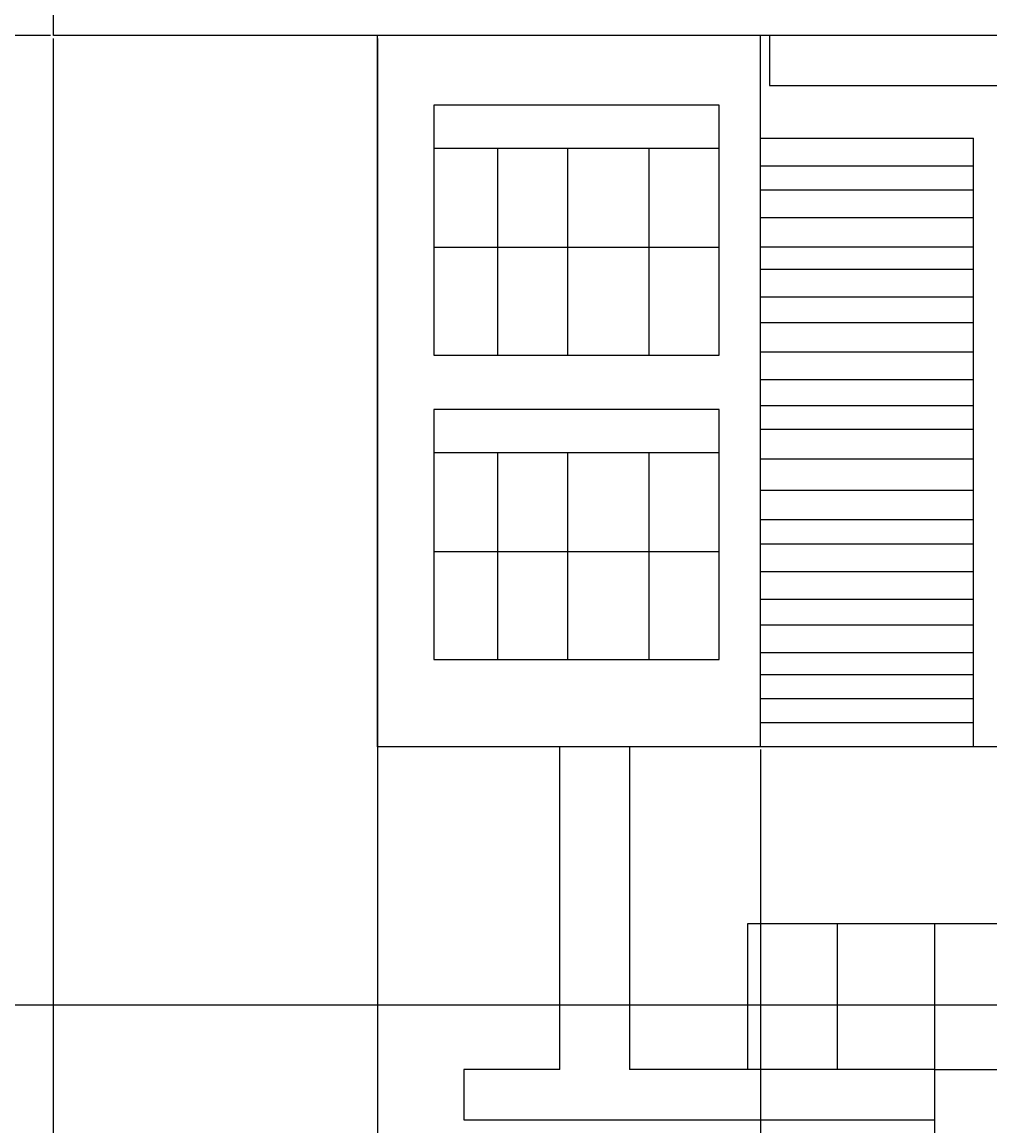
# Model space of a CAD drawing. Units: inches. Extents: x -117 to 121, y -77 to 40.
# Tile 4 of 45: x -95 to -73, y -48 to -23. Entities that reach past the tile are written whole.
import ezdxf

# ---------------------------------------------------------------- set-up
doc = ezdxf.new("R2010")
doc.units = ezdxf.units.IN
doc.header["$MEASUREMENT"] = 0
doc.layers.add('A-ANNO-DIMS', color=2, linetype='Continuous', lineweight=18)
doc.layers.add('A-ELEV', color=7, linetype='Continuous', lineweight=25)
doc.styles.get("Standard").update_dxf_attribs({"font": 'arial.ttf'})
doc.dimstyles.get("Standard").update_dxf_attribs({"dimtxt": 0.18, "dimasz": 0.18, "dimexe": 0.18, "dimexo": 0.0625, "dimgap": 0.09, "dimtad": 0, "dimtih": 1, "dimtoh": 1, "dimdec": 4, "dimzin": 0, "dimdsep": 46, "dimtxsty": 'Standard', "dimcen": 0.09, "dimadec": 0, "dimazin": 0, "dimtfac": 1, "dimtdec": 4, "dimtofl": 0, "dimtmove": 0, "dimatfit": 3, "dimfxl": 1, "dimtolj": 1, "dimtzin": 0, "dimarcsym": 0})

# ---------------------------------------------------------------- blocks, each defined once
blk = doc.blocks.new('*D5')
at = {"layer": 'A-ANNO-DIMS', "color": 0, "lineweight": -2, "transparency": 16777216}
for p, q in [((-94.436, -23.563), (-94.436, -77.193)), ((-106.034, -61.438), (-106.034, -77.193)), ((-105.854, -77.013), (-100.69, -77.013)), ((-94.616, -77.013), (-99.779, -77.013))]:
    blk.add_line(p, q, dxfattribs=at)
at = {"layer": 'A-ANNO-DIMS', "color": 0, "transparency": 16777216}
for points in [[(-105.854, -76.983), (-105.854, -77.043), (-106.034, -77.013)], [(-94.616, -76.983), (-94.616, -77.043), (-94.436, -77.013)]]:
    blk.add_solid(points, dxfattribs=at)
at = {"layer": 'Defpoints', "color": 0, "transparency": 16777216}
for p in [(-94.436, -23.501), (-106.034, -61.376), (-94.436, -77.013)]:
    blk.add_point(p, dxfattribs=at)
at = {"layer": 'A-ANNO-DIMS', "color": 0, "transparency": 16777216, "insert": (-100.235, -77.013), "char_height": 0.18, "attachment_point": 5}
blk.add_mtext('\\A1;11.598', dxfattribs=at)
blk = doc.blocks.new('*D6')
at = {"layer": 'A-ANNO-DIMS', "color": 0, "lineweight": -2, "transparency": 16777216}
for p, q in [((-94.436, -23.563), (-94.436, -77.193)), ((-77.763, -61.431), (-77.763, -77.193)), ((-94.256, -77.013), (-86.554, -77.013)), ((-77.943, -77.013), (-85.645, -77.013))]:
    blk.add_line(p, q, dxfattribs=at)
at = {"layer": 'A-ANNO-DIMS', "color": 0, "transparency": 16777216}
for points in [[(-94.256, -76.983), (-94.256, -77.043), (-94.436, -77.013)], [(-77.943, -76.983), (-77.943, -77.043), (-77.763, -77.013)]]:
    blk.add_solid(points, dxfattribs=at)
at = {"layer": 'Defpoints', "color": 0, "transparency": 16777216}
for p in [(-94.436, -23.501), (-77.763, -61.369), (-77.763, -77.013)]:
    blk.add_point(p, dxfattribs=at)
at = {"layer": 'A-ANNO-DIMS', "color": 0, "transparency": 16777216, "insert": (-86.099, -77.013), "char_height": 0.18, "attachment_point": 5}
blk.add_mtext('\\A1;16.672', dxfattribs=at)
blk = doc.blocks.new('*D13')
at = {"layer": 'A-ANNO-DIMS', "color": 0, "lineweight": -2, "transparency": 16777216}
for p, q in [((-2.663, 27.063), (-117.024, 27.063)), ((-116.844, 26.883), (-116.844, -16.974)), ((-116.844, -61.196), (-116.844, -17.338)), ((-106.096, -61.376), (-117.024, -61.376))]:
    blk.add_line(p, q, dxfattribs=at)
at = {"layer": 'A-ANNO-DIMS', "color": 0, "transparency": 16777216}
for points in [[(-116.874, 26.883), (-116.814, 26.883), (-116.844, 27.063)], [(-116.874, -61.196), (-116.814, -61.196), (-116.844, -61.376)]]:
    blk.add_solid(points, dxfattribs=at)
at = {"layer": 'Defpoints', "color": 0, "transparency": 16777216}
for p in [(-2.6, 27.063), (-116.844, -61.376), (-106.034, -61.376)]:
    blk.add_point(p, dxfattribs=at)
at = {"layer": 'A-ANNO-DIMS', "color": 0, "transparency": 16777216, "insert": (-116.844, -17.156), "char_height": 0.18, "attachment_point": 5}
blk.add_mtext('\\A1;88.44', dxfattribs=at)
blk = doc.blocks.new('*D18')
at = {"layer": 'A-ANNO-DIMS', "color": 0, "lineweight": -2, "transparency": 16777216}
for p, q in [((-94.498, -23.501), (-117.024, -23.501)), ((-116.844, -23.681), (-116.844, -42.253)), ((-116.844, -61.189), (-116.844, -42.617)), ((-77.826, -61.369), (-117.024, -61.369))]:
    blk.add_line(p, q, dxfattribs=at)
at = {"layer": 'A-ANNO-DIMS', "color": 0, "transparency": 16777216}
for points in [[(-116.874, -23.681), (-116.814, -23.681), (-116.844, -23.501)], [(-116.874, -61.189), (-116.814, -61.189), (-116.844, -61.369)]]:
    blk.add_solid(points, dxfattribs=at)
at = {"layer": 'Defpoints', "color": 0, "transparency": 16777216}
for p in [(-94.436, -23.501), (-116.844, -61.369), (-77.763, -61.369)]:
    blk.add_point(p, dxfattribs=at)
at = {"layer": 'A-ANNO-DIMS', "color": 0, "transparency": 16777216, "insert": (-116.844, -42.435), "char_height": 0.18, "attachment_point": 5}
blk.add_mtext('\\A1;37.87', dxfattribs=at)
blk = doc.blocks.new('*D19')
at = {"layer": 'A-ANNO-DIMS', "color": 0, "lineweight": -2, "transparency": 16777216}
for p, q in [((-94.498, -12.133), (-117.024, -12.133)), ((-116.844, -12.313), (-116.844, -17.635)), ((-116.844, -23.321), (-116.844, -17.999)), ((-94.498, -23.501), (-117.024, -23.501))]:
    blk.add_line(p, q, dxfattribs=at)
at = {"layer": 'A-ANNO-DIMS', "color": 0, "transparency": 16777216}
for points in [[(-116.874, -12.313), (-116.814, -12.313), (-116.844, -12.133)], [(-116.874, -23.321), (-116.814, -23.321), (-116.844, -23.501)]]:
    blk.add_solid(points, dxfattribs=at)
at = {"layer": 'Defpoints', "color": 0, "transparency": 16777216}
for p in [(-94.436, -12.133), (-116.844, -23.501), (-94.436, -23.501)]:
    blk.add_point(p, dxfattribs=at)
at = {"layer": 'A-ANNO-DIMS', "color": 0, "transparency": 16777216, "insert": (-116.844, -17.817), "char_height": 0.18, "attachment_point": 5}
blk.add_mtext('\\A1;11.367', dxfattribs=at)
blk = doc.blocks.new('*D21')
at = {"layer": 'A-ANNO-DIMS', "color": 0, "lineweight": -2, "transparency": 16777216}
for p, q in [((-106.034, -61.313), (-106.034, 38.61)), ((-75.804, 8.087), (-75.804, 38.61)), ((-105.854, 38.43), (-91.382, 38.43)), ((-75.984, 38.43), (-90.455, 38.43))]:
    blk.add_line(p, q, dxfattribs=at)
at = {"layer": 'A-ANNO-DIMS', "color": 0, "transparency": 16777216}
for points in [[(-105.854, 38.46), (-105.854, 38.4), (-106.034, 38.43)], [(-75.984, 38.46), (-75.984, 38.4), (-75.804, 38.43)]]:
    blk.add_solid(points, dxfattribs=at)
at = {"layer": 'Defpoints', "color": 0, "transparency": 16777216}
for p in [(-75.804, 38.43), (-75.804, 8.025), (-106.034, -61.376)]:
    blk.add_point(p, dxfattribs=at)
at = {"layer": 'A-ANNO-DIMS', "color": 0, "transparency": 16777216, "insert": (-90.919, 38.43), "char_height": 0.18, "attachment_point": 5}
blk.add_mtext('\\A1;30.230', dxfattribs=at)
blk = doc.blocks.new('*D37')
at = {"layer": 'A-ANNO-DIMS', "color": 0, "lineweight": -2, "transparency": 16777216}
for p, q in [((-3.912, -45.613), (-117.024, -45.613)), ((-116.844, -45.793), (-116.844, -52.47)), ((-116.844, -59.512), (-116.844, -52.834)), ((-3.912, -59.692), (-117.024, -59.692))]:
    blk.add_line(p, q, dxfattribs=at)
at = {"layer": 'A-ANNO-DIMS', "color": 0, "transparency": 16777216}
for points in [[(-116.874, -45.793), (-116.814, -45.793), (-116.844, -45.613)], [(-116.874, -59.512), (-116.814, -59.512), (-116.844, -59.692)]]:
    blk.add_solid(points, dxfattribs=at)
at = {"layer": 'Defpoints', "color": 0, "transparency": 16777216}
for p in [(-116.844, -45.613), (-3.85, -45.613), (-3.85, -59.692)]:
    blk.add_point(p, dxfattribs=at)
at = {"layer": 'A-ANNO-DIMS', "color": 0, "transparency": 16777216, "insert": (-116.844, -52.652), "char_height": 0.18, "attachment_point": 5}
blk.add_mtext('\\A1;14.079', dxfattribs=at)
blk = doc.blocks.new('*D44')
at = {"layer": 'A-ANNO-DIMS', "color": 0, "lineweight": -2, "transparency": 16777216}
for p, q in [((-94.436, -23.563), (-94.436, -77.193)), ((-87.042, -23.563), (-87.042, -77.193)), ((-94.256, -77.013), (-91.132, -77.013)), ((-87.222, -77.013), (-90.346, -77.013))]:
    blk.add_line(p, q, dxfattribs=at)
at = {"layer": 'A-ANNO-DIMS', "color": 0, "transparency": 16777216}
for points in [[(-94.256, -76.983), (-94.256, -77.043), (-94.436, -77.013)], [(-87.222, -76.983), (-87.222, -77.043), (-87.042, -77.013)]]:
    blk.add_solid(points, dxfattribs=at)
at = {"layer": 'Defpoints', "color": 0, "transparency": 16777216}
for p in [(-94.436, -23.501), (-87.042, -23.501), (-87.042, -77.013)]:
    blk.add_point(p, dxfattribs=at)
at = {"layer": 'A-ANNO-DIMS', "color": 0, "transparency": 16777216, "insert": (-90.739, -77.013), "char_height": 0.18, "attachment_point": 5}
blk.add_mtext('\\A1;7.393', dxfattribs=at)
blk = doc.blocks.new('*D45')
at = {"layer": 'A-ANNO-DIMS', "color": 0, "lineweight": -2, "transparency": 16777216}
for p, q in [((-87.042, -39.778), (-87.042, -77.193)), ((-78.307, -39.778), (-78.307, -77.193)), ((-86.862, -77.013), (-83.068, -77.013)), ((-78.487, -77.013), (-82.281, -77.013))]:
    blk.add_line(p, q, dxfattribs=at)
at = {"layer": 'A-ANNO-DIMS', "color": 0, "transparency": 16777216}
for points in [[(-86.862, -76.983), (-86.862, -77.043), (-87.042, -77.013)], [(-78.487, -76.983), (-78.487, -77.043), (-78.307, -77.013)]]:
    blk.add_solid(points, dxfattribs=at)
at = {"layer": 'Defpoints', "color": 0, "transparency": 16777216}
for p in [(-87.042, -39.716), (-78.307, -39.716), (-78.307, -77.013)]:
    blk.add_point(p, dxfattribs=at)
at = {"layer": 'A-ANNO-DIMS', "color": 0, "transparency": 16777216, "insert": (-82.675, -77.013), "char_height": 0.18, "attachment_point": 5}
blk.add_mtext('\\A1;8.736', dxfattribs=at)
blk = doc.blocks.new('*D46')
at = {"layer": 'A-ANNO-DIMS', "color": 0, "lineweight": -2, "transparency": 16777216}
for p, q in [((-78.307, -39.778), (-78.307, -77.193)), ((-72.705, -39.778), (-72.705, -77.193)), ((-78.127, -77.013), (-75.882, -77.013)), ((-72.885, -77.013), (-75.13, -77.013))]:
    blk.add_line(p, q, dxfattribs=at)
at = {"layer": 'A-ANNO-DIMS', "color": 0, "transparency": 16777216}
for points in [[(-78.127, -76.983), (-78.127, -77.043), (-78.307, -77.013)], [(-72.885, -76.983), (-72.885, -77.043), (-72.705, -77.013)]]:
    blk.add_solid(points, dxfattribs=at)
at = {"layer": 'Defpoints', "color": 0, "transparency": 16777216}
for p in [(-78.307, -39.716), (-72.705, -39.716), (-72.705, -77.013)]:
    blk.add_point(p, dxfattribs=at)
at = {"layer": 'A-ANNO-DIMS', "color": 0, "transparency": 16777216, "insert": (-75.506, -77.013), "char_height": 0.18, "attachment_point": 5}
blk.add_mtext('\\A1;5.601', dxfattribs=at)

msp = doc.modelspace()

# ---------------------------------------------------------------- linework, layer by layer
at = {"layer": 'A-ELEV'}
for p, q in [((-94.4355, -23.5007), (-94.4355, -12.1334)), ((-45.4848, -23.5007), (-94.4355, -23.5007)), ((-87.0424, -39.716), (-87.0424, -23.5007)), ((-78.3068, -39.716), (-78.3068, -23.5007)), ((-78.1044, -23.5007), (-78.1044, -24.6358)), ((-78.1044, -24.6358), (-45.4848, -24.6358)), ((-85.7569, -25.0837), (-85.7569, -30.7837)), ((-79.2538, -25.0837), (-85.7569, -25.0837)), ((-79.2538, -30.7837), (-79.2538, -25.0837)), ((-78.3068, -25.8422), (-73.4512, -25.8422)), ((-73.4512, -39.716), (-73.4512, -25.8422)), ((-79.2538, -26.0779), (-85.7569, -26.0779)), ((-84.297, -30.7837), (-84.297, -26.0779)), ((-82.7044, -30.7837), (-82.7044, -26.0779)), ((-80.8464, -30.7837), (-80.8464, -26.0779)), ((-78.3068, -26.4721), (-73.4512, -26.4721)), ((-78.3068, -27.018), (-73.4512, -27.018)), ((-78.3068, -27.648), (-73.4512, -27.648)), ((-79.2538, -28.3314), (-85.7569, -28.3314)), ((-78.3068, -28.3199), (-73.4512, -28.3199)), ((-78.3068, -28.8238), (-73.4512, -28.8238)), ((-78.3068, -29.4537), (-73.4512, -29.4537)), ((-78.3068, -30.0416), (-73.4512, -30.0416)), ((-85.7569, -30.7837), (-79.2538, -30.7837)), ((-78.3068, -30.7136), (-73.4512, -30.7136)), ((-78.3068, -31.3435), (-73.4512, -31.3435)), ((-78.3068, -31.9314), (-73.4512, -31.9314)), ((-85.7569, -32.0237), (-85.7569, -37.7236)), ((-79.2538, -32.0237), (-85.7569, -32.0237)), ((-79.2538, -37.7236), (-79.2538, -32.0237)), ((-78.3068, -32.4773), (-73.4512, -32.4773)), ((-79.2538, -33.0178), (-85.7569, -33.0178)), ((-84.297, -37.7236), (-84.297, -33.0178)), ((-82.7044, -37.7236), (-82.7044, -33.0178)), ((-80.8464, -37.7236), (-80.8464, -33.0178)), ((-78.3068, -33.1492), (-73.4512, -33.1492)), ((-78.3068, -33.8631), (-73.4512, -33.8631)), ((-78.3068, -34.5351), (-73.4512, -34.5351)), ((-78.3068, -35.0909), (-73.4512, -35.0909)), ((-79.2538, -35.2713), (-85.7569, -35.2713)), ((-78.3068, -35.7208), (-73.4512, -35.7208)), ((-78.3068, -36.3507), (-73.4512, -36.3507)), ((-78.3068, -36.9386), (-73.4512, -36.9386)), ((-85.7569, -37.7236), (-79.2538, -37.7236)), ((-78.3068, -37.5685), (-73.4512, -37.5685)), ((-78.3068, -38.0725), (-73.4512, -38.0725)), ((-78.3068, -38.6184), (-73.4512, -38.6184)), ((-78.3068, -39.1643), (-73.4512, -39.1643)), ((-63.664, -39.716), (-87.0424, -39.716)), ((-82.8832, -47.0788), (-82.8832, -39.716)), ((-81.2981, -39.716), (-81.2981, -47.0788)), ((-78.5987, -47.0788), (-78.5987, -43.7463)), ((-78.5987, -43.7463), (-74.3335, -43.7463)), ((-76.5528, -47.0788), (-76.5528, -43.7463)), ((-74.3335, -47.0788), (-74.3335, -43.7463)), ((-74.3335, -43.7463), (-46.814, -43.7463)), ((-82.8832, -47.0788), (-85.0762, -47.0788)), ((-85.0762, -47.0788), (-85.0762, -48.2271)), ((-74.3335, -47.0788), (-81.2981, -47.0788)), ((-74.3335, -47.0788), (-22.8601, -47.0788)), ((-74.3335, -54.9073), (-74.3335, -47.0788)), ((-85.0762, -48.2271), (-82.8832, -48.2271)), ((-82.8832, -48.2271), (-74.3335, -48.2271))]:
    msp.add_line(p, q, dxfattribs=at)

# ---------------------------------------------------------------- dimensions: what is measured, and where the dimension line sits
at = {"layer": 'A-ANNO-DIMS'}
for base, p1, p2, picture, middle in [((-75.8037, 38.4297), (-106.0338, -61.3756), (-75.8037, 8.0246), '*D21', (-90.9187, 38.4297)), ((-94.4355, -77.0135), (-106.0338, -61.3756), (-94.4355, -23.5007), '*D5', (-100.2346, -77.0135)), ((-77.7631, -77.0135), (-94.4355, -23.5007), (-77.7631, -61.3689), '*D6', (-86.0993, -77.0135)), ((-87.0424, -77.0135), (-94.4355, -23.5007), (-87.0424, -23.5007), '*D44', (-90.739, -77.0135)), ((-78.3068, -77.0135), (-87.0424, -39.716), (-78.3068, -39.716), '*D45', (-82.6746, -77.0135)), ((-72.70528, -77.01347), (-78.30676, -39.71597), (-72.70528, -39.71597), '*D46', (-75.50602, -77.01347))]:
    dim = msp.add_linear_dim(base=base, p1=p1, p2=p2, dimstyle='Standard', override={"dimdec": 3, "dimlfac": 1, "dimrnd": 0, "dimzin": 0, "dimdsep": 46, "dimlunit": 2}, dxfattribs=at)
    dim.commit()
    dim.dimension.update_dxf_attribs({"geometry": picture, "text_midpoint": middle})
for base, p1, p2, override, picture, middle in [((-116.8438, -61.3756), (-2.6001, 27.0634), (-106.0338, -61.3756), {"dimdec": 2, "dimlfac": 1, "dimrnd": 0, "dimzin": 0, "dimdsep": 46, "dimlunit": 2}, '*D13', (-116.8438, -17.1561)), ((-116.8438, -23.5007), (-94.4355, -12.1334), (-94.4355, -23.5007), {"dimdec": 3, "dimlfac": 1, "dimrnd": 0, "dimzin": 0, "dimdsep": 46, "dimlunit": 2}, '*D19', (-116.8438, -17.817)), ((-116.8438, -61.3689), (-94.4355, -23.5007), (-77.7631, -61.3689), {"dimdec": 2, "dimlfac": 1, "dimrnd": 0, "dimzin": 0, "dimdsep": 46, "dimlunit": 2}, '*D18', (-116.8438, -42.4348)), ((-116.843772, -45.612514), (-3.849514, -59.692012), (-3.849514, -45.612514), {"dimdec": 3, "dimlfac": 1, "dimrnd": 0, "dimzin": 0, "dimdsep": 46, "dimlunit": 2}, '*D37', (-116.843772, -52.652263))]:
    dim = msp.add_linear_dim(base=base, p1=p1, p2=p2, angle=90, dimstyle='Standard', override=override, dxfattribs=at)
    dim.commit()
    dim.dimension.update_dxf_attribs({"geometry": picture, "text_midpoint": middle})

doc.saveas('drawing.dxf')
